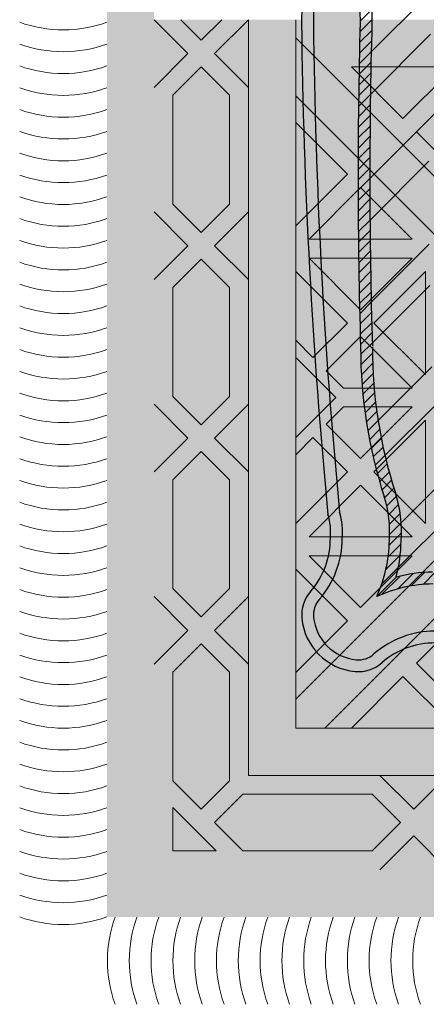
# Model space of a CAD drawing. Units: inches. Extents: x 844 to 2234, y 346 to 1084.
# Tile 52 of 93: x 1861.15 to 1866.64, y 688.07 to 701.36. Entities that reach past the tile are written whole.
import ezdxf

# ---------------------------------------------------------------- set-up
doc = ezdxf.new("R2010")
doc.units = ezdxf.units.IN
doc.header["$MEASUREMENT"] = 0
doc.layers.add('furniture', color=8, linetype='Continuous', lineweight=18)
doc.layers.add('RA-AP-01$0$INT', color=35, linetype='Continuous', lineweight=5)
doc.layers.add('RA-AP-01$0$FURN', color=3, linetype='Continuous')
doc.layers.add('RA-AP-01$0$WOOD', color=64, linetype='Continuous')

# ---------------------------------------------------------------- blocks, each defined once
blk = doc.blocks.new('A$C18D01794')
at = {"layer": 'RA-AP-01$0$INT'}
h = blk.add_hatch(color=256, dxfattribs=at)
h.paths.add_polyline_path([(4.3552, -6.1567), (4.3552, -8.0567), (5.4552, -8.0567), (5.4552, -6.1567)])
h.paths.add_polyline_path([(4.4052, -8.0067), (4.4052, -6.2067), (5.4052, -6.2067), (5.4052, -8.0067)], flags=16)
h = blk.add_hatch(color=256, dxfattribs=at)
h.paths.add_polyline_path([(4.4693, -7.0709), (4.5052, -7.035), (4.5052, -7.1067)])
h.paths.add_polyline_path([(4.4552, -7.085), (4.4769, -7.1067), (4.4335, -7.1067)])
h.paths.add_polyline_path([(4.4052, -7.035), (4.4411, -7.0709), (4.4052, -7.1067)])
h.paths.add_polyline_path([(4.4252, -6.9115), (4.4552, -6.8815), (4.4852, -6.9115), (4.4852, -7.0267), (4.4552, -7.0567), (4.4252, -7.0267)])
h.paths.add_polyline_path([(4.5052, -6.8315), (4.5052, -6.9032), (4.4693, -6.8673)])
h.paths.add_polyline_path([(4.4252, -6.7079), (4.4552, -6.6779), (4.4852, -6.7079), (4.4852, -6.8232), (4.4552, -6.8532), (4.4252, -6.8232)])
h.paths.add_polyline_path([(4.4252, -6.5044), (4.4552, -6.4744), (4.4852, -6.5044), (4.4852, -6.6196), (4.4552, -6.6496), (4.4252, -6.6196)])
h.paths.add_polyline_path([(4.4693, -6.6638), (4.5052, -6.6279), (4.5052, -6.6996)])
h.paths.add_polyline_path([(4.4052, -6.6279), (4.4411, -6.6638), (4.4052, -6.6996)])
h.paths.add_polyline_path([(4.4052, -6.4244), (4.4411, -6.4602), (4.4052, -6.4961)])
h.paths.add_polyline_path([(4.4693, -6.4602), (4.5052, -6.4244), (4.5052, -6.4961)])
h.paths.add_polyline_path([(4.4252, -6.3009), (4.4552, -6.2709), (4.4852, -6.3009), (4.4852, -6.4161), (4.4552, -6.4461), (4.4252, -6.4161)])
h.paths.add_polyline_path([(4.4252, -6.2267), (4.4711, -6.2267), (4.4252, -6.2726)])
h.paths.add_polyline_path([(4.4993, -6.2267), (4.6361, -6.2267), (4.6661, -6.2567), (4.6361, -6.2867), (4.4993, -6.2867), (4.4693, -6.2567)])
h.paths.add_polyline_path([(4.6802, -6.2709), (4.7161, -6.3067), (4.6443, -6.3067)])
h.paths.add_polyline_path([(4.6443, -6.2067), (4.7161, -6.2067), (4.6802, -6.2426)])
h.paths.add_polyline_path([(4.7243, -6.2267), (4.8611, -6.2267), (4.8911, -6.2567), (4.8611, -6.2867), (4.7243, -6.2867), (4.6943, -6.2567)])
h.paths.add_polyline_path([(4.9052, -6.2709), (4.9411, -6.3067), (4.8693, -6.3067)])
h.paths.add_polyline_path([(4.8693, -6.2067), (4.9411, -6.2067), (4.9052, -6.2426)])
h.paths.add_polyline_path([(4.9493, -6.2267), (5.0861, -6.2267), (5.1161, -6.2567), (5.0861, -6.2867), (4.9493, -6.2867), (4.9193, -6.2567)])
h.paths.add_polyline_path([(5.1302, -6.2709), (5.1661, -6.3067), (5.0943, -6.3067)])
h.paths.add_polyline_path([(5.0943, -6.2067), (5.1661, -6.2067), (5.1302, -6.2426)])
h.paths.add_polyline_path([(5.1743, -6.2267), (5.3111, -6.2267), (5.3411, -6.2567), (5.3111, -6.2867), (5.1743, -6.2867), (5.1443, -6.2567)])
h.paths.add_polyline_path([(5.3252, -6.3009), (5.3552, -6.2709), (5.3852, -6.3009), (5.3852, -6.4161), (5.3552, -6.4461), (5.3252, -6.4161)])
h.paths.add_polyline_path([(5.3393, -6.2267), (5.3852, -6.2267), (5.3852, -6.2726)])
h.paths.add_polyline_path([(5.3252, -6.5044), (5.3552, -6.4744), (5.3852, -6.5044), (5.3852, -6.6196), (5.3552, -6.6496), (5.3252, -6.6196)])
h.paths.add_polyline_path([(5.3052, -6.4244), (5.3411, -6.4602), (5.3052, -6.4961)])
h.paths.add_polyline_path([(5.3693, -6.4602), (5.4052, -6.4244), (5.4052, -6.4961)])
h.paths.add_polyline_path([(5.4052, -6.6279), (5.4052, -6.6996), (5.3693, -6.6638)])
h.paths.add_polyline_path([(5.3052, -6.6279), (5.3411, -6.6638), (5.3052, -6.6996)])
h.paths.add_polyline_path([(5.3252, -6.7079), (5.3552, -6.6779), (5.3852, -6.7079), (5.3852, -6.8232), (5.3552, -6.8532), (5.3252, -6.8232)])
h.paths.add_polyline_path([(5.3052, -6.8315), (5.3411, -6.8673), (5.3052, -6.9032)])
h.paths.add_polyline_path([(5.3252, -6.9115), (5.3552, -6.8815), (5.3852, -6.9115), (5.3852, -7.0267), (5.3552, -7.0567), (5.3252, -7.0267)])
h.paths.add_polyline_path([(5.4046, -6.8321, 0.001218), (5.4052, -6.8323), (5.4052, -6.9032), (5.3693, -6.8673)])
h.paths.add_polyline_path([(5.3693, -7.0709), (5.4052, -7.035), (5.4052, -7.1067)])
h.paths.add_polyline_path([(5.3552, -7.085), (5.3769, -7.1067), (5.3335, -7.1067)])
h.paths.add_polyline_path([(5.3052, -7.035), (5.3411, -7.0709), (5.3052, -7.1067)])
h = blk.add_hatch(color=256, dxfattribs=at)
h.paths.add_polyline_path([(4.5052, -6.6279), (4.4693, -6.6638), (4.5052, -6.6996), (4.5052, -6.8315), (4.4693, -6.8673), (4.5052, -6.9032), (4.5052, -7.035), (4.4693, -7.0709), (4.5052, -7.1067), (4.4769, -7.1067), (4.4552, -7.085), (4.4335, -7.1067), (4.4052, -7.1067), (4.4411, -7.0709), (4.4052, -7.035), (4.4052, -6.9032), (4.4411, -6.8673), (4.4052, -6.8315), (4.4052, -6.6996), (4.4411, -6.6638), (4.4052, -6.6279), (4.4052, -6.4961), (4.4411, -6.4602), (4.4052, -6.4244), (4.4052, -6.2067), (4.6443, -6.2067), (4.6802, -6.2426), (4.7161, -6.2067), (4.8693, -6.2067), (4.9052, -6.2426), (4.9411, -6.2067), (5.0943, -6.2067), (5.1302, -6.2426), (5.1661, -6.2067), (5.4052, -6.2067), (5.4052, -6.4244), (5.3693, -6.4602), (5.4052, -6.4961), (5.4052, -6.6279), (5.3693, -6.6638), (5.4052, -6.6996), (5.4052, -6.8315), (5.3693, -6.8673), (5.4052, -6.9032), (5.4052, -7.035), (5.3693, -7.0709), (5.4052, -7.1067), (5.3769, -7.1067), (5.3552, -7.085), (5.3335, -7.1067), (5.3052, -7.1067), (5.3411, -7.0709), (5.3052, -7.035), (5.3052, -6.9032), (5.3411, -6.8673), (5.3052, -6.8315), (5.3052, -6.6996), (5.3411, -6.6638), (5.3052, -6.6279), (5.3052, -6.4961), (5.3411, -6.4602), (5.3052, -6.4244), (5.3052, -6.3067), (5.1661, -6.3067), (5.1302, -6.2709), (5.0943, -6.3067), (4.9411, -6.3067), (4.9052, -6.2709), (4.8693, -6.3067), (4.7161, -6.3067), (4.6802, -6.2709), (4.6443, -6.3067), (4.5052, -6.3067), (4.5052, -6.4244), (4.4693, -6.4602), (4.5052, -6.4961)])
h.paths.add_polyline_path([(4.4852, -6.5044), (4.4552, -6.4744), (4.4252, -6.5044), (4.4252, -6.6196), (4.4552, -6.6496), (4.4852, -6.6196)], flags=16)
h.paths.add_polyline_path([(4.4552, -6.4461), (4.4852, -6.4161), (4.4852, -6.3009), (4.4552, -6.2709), (4.4252, -6.3009), (4.4252, -6.4161)], flags=16)
h.paths.add_polyline_path([(4.4552, -6.6779), (4.4252, -6.7079), (4.4252, -6.8232), (4.4552, -6.8532), (4.4852, -6.8232), (4.4852, -6.7079)], flags=16)
h.paths.add_polyline_path([(4.4993, -6.2867), (4.6361, -6.2867), (4.6661, -6.2567), (4.6361, -6.2267), (4.4993, -6.2267), (4.4693, -6.2567)], flags=16)
h.paths.add_polyline_path([(4.4252, -6.2726), (4.4711, -6.2267), (4.4252, -6.2267)], flags=16)
h.paths.add_polyline_path([(4.4552, -6.8815), (4.4252, -6.9115), (4.4252, -7.0267), (4.4552, -7.0567), (4.4852, -7.0267), (4.4852, -6.9115)], flags=16)
h.paths.add_polyline_path([(4.7243, -6.2867), (4.8611, -6.2867), (4.8911, -6.2567), (4.8611, -6.2267), (4.7243, -6.2267), (4.6943, -6.2567)], flags=16)
h.paths.add_polyline_path([(4.9193, -6.2567), (4.9493, -6.2867), (5.0861, -6.2867), (5.1161, -6.2567), (5.0861, -6.2267), (4.9493, -6.2267)], flags=16)
h.paths.add_polyline_path([(5.1443, -6.2567), (5.1743, -6.2867), (5.3111, -6.2867), (5.3411, -6.2567), (5.3111, -6.2267), (5.1743, -6.2267)], flags=16)
h.paths.add_polyline_path([(5.3252, -6.6196), (5.3552, -6.6496), (5.3852, -6.6196), (5.3852, -6.5044), (5.3552, -6.4744), (5.3252, -6.5044)], flags=16)
h.paths.add_polyline_path([(5.3252, -6.4161), (5.3552, -6.4461), (5.3852, -6.4161), (5.3852, -6.3009), (5.3552, -6.2709), (5.3252, -6.3009)], flags=16)
h.paths.add_polyline_path([(5.3252, -6.7079), (5.3252, -6.8232), (5.3552, -6.8532), (5.3852, -6.8232), (5.3852, -6.7079), (5.3552, -6.6779)], flags=16)
h.paths.add_polyline_path([(5.3252, -6.9115), (5.3252, -7.0267), (5.3552, -7.0567), (5.3852, -7.0267), (5.3852, -6.9115), (5.3552, -6.8815)], flags=16)
h.paths.add_polyline_path([(5.3393, -6.2267), (5.3852, -6.2726), (5.3852, -6.2267)], flags=16)
for points in [[(4.5052, -6.3067), (5.3052, -6.3067), (5.3052, -7.1067), (5.2552, -7.1067), (5.2552, -6.3567), (4.5552, -6.3567), (4.5552, -7.1067), (4.5052, -7.1067)], [(4.4052, -6.9032), (4.4411, -6.8673), (4.4052, -6.8315)]]:
    blk.add_hatch(color=256, dxfattribs=at).paths.add_polyline_path(points)
h = blk.add_hatch(color=256, dxfattribs=at)
h.paths.add_polyline_path([(4.5859, -6.3567), (4.5552, -6.3567), (4.5552, -6.3874), (4.8745, -6.7067), (4.9052, -6.676)])
h.paths.add_polyline_path([(5.2552, -6.3874), (5.2552, -6.3567), (5.2245, -6.3567), (4.9052, -6.676), (4.9359, -6.7067)])
h.paths.add_polyline_path([(4.9359, -6.7067), (4.9052, -6.7374), (5.2552, -7.0874), (5.2552, -7.026)])
h.paths.add_polyline_path([(4.5552, -7.026), (4.5552, -7.0874), (4.9052, -6.7374), (4.8745, -6.7067)])
h = blk.add_hatch(color=256, dxfattribs=at)
h.paths.add_polyline_path([(4.5859, -6.3567), (4.6142, -6.3567), (4.6688, -6.4114), (4.7235, -6.3567), (4.7718, -6.3567), (4.8264, -6.4114), (4.8628, -6.375), (4.8445, -6.3567), (4.8628, -6.3567), (4.9052, -6.3991), (4.9476, -6.3567), (4.9659, -6.3567), (4.9476, -6.375), (4.984, -6.4114), (5.0386, -6.3567), (5.0869, -6.3567), (5.1416, -6.4114), (5.1962, -6.3567), (5.2245, -6.3567), (4.9052, -6.676)])
h.paths.add_polyline_path([(4.8952, -6.6377), (4.8952, -6.5284), (4.8406, -6.5831)], flags=16)
h.paths.add_polyline_path([(4.9152, -6.6377), (4.9699, -6.5831), (4.9152, -6.5284)], flags=16)
h.paths.add_polyline_path([(4.8264, -6.5689), (4.8811, -6.5143), (4.7718, -6.5143)], flags=16)
h.paths.add_polyline_path([(4.984, -6.5689), (5.0386, -6.5143), (4.9293, -6.5143)], flags=16)
h.paths.add_polyline_path([(4.8811, -6.4943), (4.8264, -6.4396), (4.7718, -6.4943)], flags=16)
h.paths.add_polyline_path([(4.9293, -6.4943), (5.0386, -6.4943), (4.984, -6.4396)], flags=16)
h.paths.add_polyline_path([(4.8952, -6.4801), (4.8952, -6.4074), (4.8769, -6.3891), (4.8406, -6.4255)], flags=16)
h.paths.add_polyline_path([(4.9152, -6.4801), (4.9699, -6.4255), (4.9335, -6.3891), (4.9152, -6.4074)], flags=16)
h.paths.add_polyline_path([(4.7576, -6.4801), (4.8123, -6.4255), (4.7576, -6.3709)], flags=16)
h.paths.add_polyline_path([(4.7376, -6.4801), (4.7376, -6.3709), (4.683, -6.4255)], flags=16)
h.paths.add_polyline_path([(5.0528, -6.4801), (5.0528, -6.3709), (4.9981, -6.4255)], flags=16)
h.paths.add_polyline_path([(5.0728, -6.4801), (5.1274, -6.4255), (5.0728, -6.3709)], flags=16)
h.paths.add_polyline_path([(4.9359, -6.7067), (5.2552, -6.3874), (5.2552, -6.4157), (5.2006, -6.4704), (5.2552, -6.525), (5.2552, -6.5733), (5.2006, -6.6279), (5.2369, -6.6643), (5.2552, -6.646), (5.2552, -6.6643), (5.2128, -6.7067), (5.2552, -6.7491), (5.2552, -6.7674), (5.2369, -6.7491), (5.2006, -6.7855), (5.2552, -6.8401), (5.2552, -6.8884), (5.2006, -6.9431), (5.2552, -6.9977), (5.2552, -7.026)])
h.paths.add_polyline_path([(5.043, -6.7855), (5.0976, -6.8401), (5.0976, -6.7309)], flags=16)
h.paths.add_polyline_path([(5.0288, -6.7714), (5.0835, -6.7167), (4.9742, -6.7167)], flags=16)
h.paths.add_polyline_path([(5.1176, -6.8401), (5.1723, -6.7855), (5.1176, -6.7309)], flags=16)
h.paths.add_polyline_path([(5.0835, -6.6967), (5.0288, -6.6421), (4.9742, -6.6967)], flags=16)
h.paths.add_polyline_path([(5.1318, -6.8543), (5.1864, -6.7996), (5.2411, -6.8543)], flags=17)
h.paths.add_polyline_path([(5.1318, -6.7167), (5.1864, -6.7714), (5.2228, -6.735), (5.2045, -6.7167)], flags=16)
h.paths.add_polyline_path([(5.0976, -6.6826), (5.0976, -6.5733), (5.043, -6.6279)], flags=16)
h.paths.add_polyline_path([(5.1318, -6.8743), (5.2411, -6.8743), (5.1864, -6.9289)], flags=17)
h.paths.add_polyline_path([(5.1318, -6.6967), (5.2045, -6.6967), (5.2228, -6.6784), (5.1864, -6.6421)], flags=16)
h.paths.add_polyline_path([(5.1176, -6.6826), (5.1723, -6.6279), (5.1176, -6.5733)], flags=16)
h.paths.add_polyline_path([(5.1864, -6.6138), (5.2411, -6.5591), (5.1318, -6.5591)], flags=16)
h.paths.add_polyline_path([(5.1318, -6.5391), (5.2411, -6.5391), (5.1864, -6.4845)], flags=16)
h.paths.add_polyline_path([(5.2552, -7.0874), (5.2552, -7.1067), (4.5552, -7.1067), (4.5552, -7.0874), (4.9052, -6.7374)])
h.paths.add_polyline_path([(4.984, -6.8445), (4.9293, -6.8991), (5.0386, -6.8991)], flags=16)
h.paths.add_polyline_path([(4.9699, -6.8304), (4.9152, -6.7757), (4.9152, -6.885)], flags=16)
h.paths.add_polyline_path([(4.9293, -6.9191), (4.984, -6.9738), (5.0386, -6.9191)], flags=16)
h.paths.add_polyline_path([(5.0528, -6.9333), (4.9981, -6.9879), (5.0528, -7.0426)], flags=16)
h.paths.add_polyline_path([(5.0728, -6.9333), (5.0728, -7.0426), (5.1274, -6.9879)], flags=16)
h.paths.add_polyline_path([(4.8952, -6.7757), (4.8406, -6.8304), (4.8952, -6.885)], flags=16)
h.paths.add_polyline_path([(4.9152, -6.9333), (4.9152, -7.006), (4.9335, -7.0243), (4.9699, -6.9879)], flags=16)
h.paths.add_polyline_path([(4.8811, -6.8991), (4.8264, -6.8445), (4.7718, -6.8991)], flags=16)
h.paths.add_polyline_path([(4.8952, -6.9333), (4.8406, -6.9879), (4.8769, -7.0243), (4.8952, -7.006)], flags=16)
h.paths.add_polyline_path([(4.984, -7.0021), (4.9476, -7.0384), (4.9659, -7.0567), (5.0386, -7.0567)], flags=16)
h.paths.add_polyline_path([(4.8811, -6.9191), (4.7718, -6.9191), (4.8264, -6.9738)], flags=16)
h.paths.add_polyline_path([(4.9052, -7.0143), (4.8628, -7.0567), (4.9476, -7.0567)], flags=16)
h.paths.add_polyline_path([(5.1416, -7.0021), (5.0869, -7.0567), (5.1962, -7.0567)], flags=16)
h.paths.add_polyline_path([(4.8264, -7.0021), (4.7718, -7.0567), (4.8445, -7.0567), (4.8628, -7.0384)], flags=16)
h.paths.add_polyline_path([(4.8123, -6.9879), (4.7576, -6.9333), (4.7576, -7.0426)], flags=16)
h.paths.add_polyline_path([(4.7376, -6.9333), (4.683, -6.9879), (4.7376, -7.0426)], flags=16)
h.paths.add_polyline_path([(4.7235, -7.0567), (4.6688, -7.0021), (4.6142, -7.0567)], flags=16)
h.paths.add_polyline_path([(4.5976, -6.7067), (4.5552, -6.6643), (4.5552, -6.646), (4.5735, -6.6643), (4.6099, -6.6279), (4.5552, -6.5733), (4.5552, -6.525), (4.6099, -6.4704), (4.5552, -6.4157), (4.5552, -6.3874), (4.8745, -6.7067), (4.5552, -7.026), (4.5552, -6.9977), (4.6099, -6.9431), (4.5552, -6.8884), (4.5552, -6.8401), (4.6099, -6.7855), (4.5735, -6.7491), (4.5552, -6.7674), (4.5552, -6.7491)])
h.paths.add_polyline_path([(4.7128, -6.7309), (4.7128, -6.8401), (4.7674, -6.7855)], flags=16)
h.paths.add_polyline_path([(4.7269, -6.7167), (4.7816, -6.7714), (4.8362, -6.7167)], flags=16)
h.paths.add_polyline_path([(4.6928, -6.7309), (4.6381, -6.7855), (4.6928, -6.8401)], flags=16)
h.paths.add_polyline_path([(4.7269, -6.6967), (4.8362, -6.6967), (4.7816, -6.6421)], flags=16)
h.paths.add_polyline_path([(4.6786, -6.7167), (4.6059, -6.7167), (4.5876, -6.735), (4.624, -6.7714)], flags=16)
h.paths.add_polyline_path([(4.7128, -6.6826), (4.7674, -6.6279), (4.7128, -6.5733)], flags=16)
h.paths.add_polyline_path([(4.6786, -6.6967), (4.624, -6.6421), (4.5876, -6.6784), (4.6059, -6.6967)], flags=16)
h.paths.add_polyline_path([(4.6928, -6.6826), (4.6928, -6.5733), (4.6381, -6.6279)], flags=16)
h.paths.add_polyline_path([(4.624, -6.7996), (4.6786, -6.8543), (4.5693, -6.8543)], flags=17)
h.paths.add_polyline_path([(4.624, -6.6138), (4.6786, -6.5591), (4.5693, -6.5591)], flags=16)
h.paths.add_polyline_path([(4.6786, -6.8743), (4.624, -6.9289), (4.5693, -6.8743)], flags=17)
h.paths.add_polyline_path([(4.6786, -6.5391), (4.624, -6.4845), (4.5693, -6.5391)], flags=16)
h = blk.add_hatch(color=256, dxfattribs=at)
h.paths.add_polyline_path([(4.9699, -6.5831), (4.9152, -6.6377), (4.9152, -6.5284)])
h.paths.add_polyline_path([(4.8952, -6.6377), (4.8406, -6.5831), (4.8952, -6.5284)])
h.paths.add_polyline_path([(4.8264, -6.5689), (4.7718, -6.5143), (4.8811, -6.5143)])
h.paths.add_polyline_path([(4.8811, -6.4943), (4.7718, -6.4943), (4.8264, -6.4396)])
h.paths.add_polyline_path([(4.8952, -6.4801), (4.8406, -6.4255), (4.8769, -6.3891), (4.8952, -6.4074)])
h.paths.add_polyline_path([(4.8628, -6.375), (4.8264, -6.4114), (4.7718, -6.3567), (4.8445, -6.3567)])
h.paths.add_polyline_path([(4.8123, -6.4255), (4.7576, -6.4801), (4.7576, -6.3709)])
h.paths.add_polyline_path([(4.7376, -6.4801), (4.683, -6.4255), (4.7376, -6.3709)])
h.paths.add_polyline_path([(4.6688, -6.4114), (4.6142, -6.3567), (4.7235, -6.3567)])
h.paths.add_polyline_path([(4.9052, -6.3991), (4.8628, -6.3567), (4.9476, -6.3567)])
h.paths.add_polyline_path([(4.9152, -6.4801), (4.9152, -6.4074), (4.9335, -6.3891), (4.9699, -6.4255)])
h.paths.add_polyline_path([(5.0386, -6.4943), (4.9293, -6.4943), (4.984, -6.4396)])
h.paths.add_polyline_path([(4.984, -6.5689), (4.9293, -6.5143), (5.0386, -6.5143)])
h.paths.add_polyline_path([(5.0528, -6.4801), (4.9981, -6.4255), (5.0528, -6.3709)])
h.paths.add_polyline_path([(4.984, -6.4114), (4.9476, -6.375), (4.9659, -6.3567), (5.0386, -6.3567)])
h.paths.add_polyline_path([(5.1274, -6.4255), (5.0728, -6.4801), (5.0728, -6.3709)])
h.paths.add_polyline_path([(5.1416, -6.4114), (5.0869, -6.3567), (5.1962, -6.3567)])
h = blk.add_hatch(color=256, dxfattribs=at)
h.paths.add_polyline_path([(4.7816, -6.7714), (4.8362, -6.7167), (4.7269, -6.7167)])
h.paths.add_polyline_path([(4.8362, -6.6967), (4.7816, -6.6421), (4.7269, -6.6967)])
h.paths.add_polyline_path([(4.7674, -6.6279), (4.7128, -6.5733), (4.7128, -6.6826)])
h.paths.add_polyline_path([(4.6928, -6.6826), (4.6928, -6.5733), (4.6381, -6.6279)])
h.paths.add_polyline_path([(4.6786, -6.6967), (4.624, -6.6421), (4.5876, -6.6784), (4.6059, -6.6967)])
h.paths.add_polyline_path([(4.5735, -6.6643), (4.6099, -6.6279), (4.5552, -6.5733), (4.5552, -6.646)])
h.paths.add_polyline_path([(4.624, -6.6138), (4.6786, -6.5591), (4.5693, -6.5591)])
h.paths.add_polyline_path([(4.6786, -6.5391), (4.624, -6.4845), (4.5693, -6.5391)])
h.paths.add_polyline_path([(4.6099, -6.4704), (4.5552, -6.4157), (4.5552, -6.525)])
h.paths.add_polyline_path([(4.5976, -6.7067), (4.5552, -6.6643), (4.5552, -6.7491)])
h.paths.add_polyline_path([(4.6786, -6.7167), (4.6059, -6.7167), (4.5876, -6.735), (4.624, -6.7714)])
h.paths.add_polyline_path([(4.6928, -6.8401), (4.6928, -6.7309), (4.6381, -6.7855)])
h.paths.add_polyline_path([(4.7674, -6.7855), (4.7128, -6.7309), (4.7128, -6.8401)])
h.paths.add_polyline_path([(4.6786, -6.8543), (4.624, -6.7996), (4.5693, -6.8543)])
h.paths.add_polyline_path([(4.6099, -6.7855), (4.5735, -6.7491), (4.5552, -6.7674), (4.5552, -6.8401)])
h.paths.add_polyline_path([(4.624, -6.9289), (4.6786, -6.8743), (4.5693, -6.8743)])
h.paths.add_polyline_path([(4.6099, -6.9431), (4.5552, -6.8884), (4.5552, -6.9977)])
h = blk.add_hatch(color=256, dxfattribs=at)
h.paths.add_polyline_path([(4.8952, -6.7757), (4.8406, -6.8304), (4.8952, -6.885)])
h.paths.add_polyline_path([(4.9152, -6.885), (4.9699, -6.8304), (4.9152, -6.7757)])
h.paths.add_polyline_path([(5.0386, -6.8991), (4.984, -6.8445), (4.9293, -6.8991)])
h.paths.add_polyline_path([(4.9293, -6.9191), (4.984, -6.9738), (5.0386, -6.9191)])
h.paths.add_polyline_path([(4.9152, -6.9333), (4.9152, -7.006), (4.9335, -7.0243), (4.9699, -6.9879)])
h.paths.add_polyline_path([(5.0386, -7.0567), (4.984, -7.0021), (4.9476, -7.0384), (4.9659, -7.0567)])
h.paths.add_polyline_path([(5.0528, -7.0426), (5.0528, -6.9333), (4.9981, -6.9879)])
h.paths.add_polyline_path([(5.0728, -7.0426), (5.1274, -6.9879), (5.0728, -6.9333)])
h.paths.add_polyline_path([(5.1416, -7.0021), (5.0869, -7.0567), (5.1962, -7.0567)])
h.paths.add_polyline_path([(4.9476, -7.0567), (4.9052, -7.0143), (4.8628, -7.0567)])
h.paths.add_polyline_path([(4.8406, -6.9879), (4.8769, -7.0243), (4.8952, -7.006), (4.8952, -6.9333)])
h.paths.add_polyline_path([(4.8811, -6.9191), (4.7718, -6.9191), (4.8264, -6.9738)])
h.paths.add_polyline_path([(4.8811, -6.8991), (4.8264, -6.8445), (4.7718, -6.8991)])
h.paths.add_polyline_path([(4.7576, -7.0426), (4.8123, -6.9879), (4.7576, -6.9333)])
h.paths.add_polyline_path([(4.8264, -7.0021), (4.7718, -7.0567), (4.8445, -7.0567), (4.8628, -7.0384)])
h.paths.add_polyline_path([(4.7376, -7.0426), (4.7376, -6.9333), (4.683, -6.9879)])
h.paths.add_polyline_path([(4.6688, -7.0021), (4.6142, -7.0567), (4.7235, -7.0567)])
for p, q in [((4.6443, -6.2067), (4.6802, -6.2426)), ((4.7161, -6.2067), (4.6802, -6.2426)), ((4.4711, -6.2267), (4.4252, -6.2726)), ((4.4252, -6.2726), (4.4252, -6.2267)), ((4.4711, -6.2267), (4.4252, -6.2267)), ((4.4993, -6.2267), (4.4693, -6.2567)), ((4.6361, -6.2267), (4.4993, -6.2267)), ((4.6361, -6.2267), (4.6661, -6.2567)), ((4.4993, -6.2867), (4.4693, -6.2567)), ((4.6361, -6.2867), (4.6661, -6.2567)), ((4.4252, -6.3009), (4.4552, -6.2709)), ((4.4852, -6.3009), (4.4552, -6.2709)), ((4.6443, -6.3067), (4.6802, -6.2709)), ((4.7161, -6.3067), (4.6802, -6.2709)), ((4.6361, -6.2867), (4.4993, -6.2867)), ((4.4252, -6.4161), (4.4252, -6.3009)), ((4.4852, -6.3009), (4.4852, -6.4161)), ((5.2672, -6.3067), (4.5432, -6.3067)), ((5.2672, -6.3067), (4.5432, -6.3067)), ((4.5552, -6.3567), (5.2552, -6.3567)), ((4.5552, -7.1067), (4.5552, -6.3567)), ((4.9052, -6.676), (4.5859, -6.3567)), ((4.6142, -6.3567), (4.6688, -6.4114)), ((4.7235, -6.3567), (4.6688, -6.4114)), ((4.7376, -6.3709), (4.683, -6.4255)), ((4.8745, -6.7067), (4.5552, -6.3874)), ((4.4552, -6.4461), (4.4252, -6.4161)), ((4.4552, -6.4461), (4.4852, -6.4161)), ((4.5552, -6.4157), (4.6099, -6.4704)), ((4.4411, -6.4602), (4.4052, -6.4244)), ((4.4693, -6.4602), (4.5052, -6.4244)), ((4.683, -6.4255), (4.7376, -6.4801)), ((4.4052, -6.4961), (4.4411, -6.4602)), ((4.5052, -6.4961), (4.4693, -6.4602)), ((4.5552, -6.525), (4.6099, -6.4704)), ((4.4252, -6.5044), (4.4552, -6.4744)), ((4.4852, -6.5044), (4.4552, -6.4744)), ((4.5693, -6.5391), (4.624, -6.4845)), ((4.624, -6.4845), (4.6786, -6.5391)), ((4.4252, -6.6196), (4.4252, -6.5044)), ((4.4852, -6.6196), (4.4852, -6.5044)), ((4.6786, -6.5391), (4.5693, -6.5391)), ((4.5693, -6.5591), (4.624, -6.6138)), ((4.6786, -6.5591), (4.5693, -6.5591)), ((4.6786, -6.5591), (4.624, -6.6138)), ((4.5552, -6.646), (4.5552, -6.5733)), ((4.5552, -6.5733), (4.6099, -6.6279)), ((4.6928, -6.5733), (4.6381, -6.6279)), ((4.6928, -6.5733), (4.6928, -6.6826)), ((4.4052, -6.6279), (4.4411, -6.6638)), ((4.4252, -6.6196), (4.4552, -6.6496)), ((4.4852, -6.6196), (4.4552, -6.6496)), ((4.5052, -6.6279), (4.4693, -6.6638)), ((4.6099, -6.6279), (4.5735, -6.6643)), ((4.6928, -6.6826), (4.6381, -6.6279)), ((4.5552, -6.646), (4.5735, -6.6643)), ((4.624, -6.6421), (4.5876, -6.6784)), ((4.6786, -6.6967), (4.624, -6.6421)), ((4.4052, -6.6996), (4.4411, -6.6638)), ((4.5052, -6.6996), (4.4693, -6.6638)), ((4.5552, -6.7491), (4.5552, -6.6643)), ((4.5976, -6.7067), (4.5552, -6.6643)), ((4.4252, -6.7079), (4.4552, -6.6779)), ((4.4852, -6.7079), (4.4552, -6.6779)), ((4.6059, -6.6967), (4.5876, -6.6784)), ((4.6059, -6.6967), (4.6786, -6.6967)), ((4.4252, -6.8232), (4.4252, -6.7079)), ((4.4852, -6.8232), (4.4852, -6.7079)), ((4.8745, -6.7067), (4.5552, -7.026)), ((4.5976, -6.7067), (4.5552, -6.7491)), ((4.6059, -6.7167), (4.5876, -6.735)), ((4.6059, -6.7167), (4.6786, -6.7167)), ((4.6786, -6.7167), (4.624, -6.7714)), ((4.6928, -6.7309), (4.6381, -6.7855)), ((4.6928, -6.8401), (4.6928, -6.7309)), ((4.9052, -6.7374), (4.5552, -7.0874)), ((4.624, -6.7714), (4.5876, -6.735)), ((4.5735, -6.7491), (4.5552, -6.7674)), ((4.5552, -6.7674), (4.5735, -6.7491)), ((4.6099, -6.7855), (4.5735, -6.7491)), ((4.5552, -6.7674), (4.5552, -6.8401)), ((4.5552, -6.8401), (4.6099, -6.7855)), ((4.6928, -6.8401), (4.6381, -6.7855)), ((4.5693, -6.8543), (4.624, -6.7996)), ((4.6786, -6.8543), (4.624, -6.7996)), ((4.4252, -6.8232), (4.4552, -6.8532)), ((4.4852, -6.8232), (4.4552, -6.8532)), ((4.4052, -6.8315), (4.4411, -6.8673)), ((4.5052, -6.8315), (4.4693, -6.8673)), ((4.6786, -6.8543), (4.5693, -6.8543)), ((4.4052, -6.9032), (4.4411, -6.8673)), ((4.5052, -6.9032), (4.4693, -6.8673)), ((4.5693, -6.8743), (4.624, -6.9289)), ((4.6786, -6.8743), (4.5693, -6.8743)), ((4.624, -6.9289), (4.6786, -6.8743)), ((4.4252, -6.9115), (4.4552, -6.8815)), ((4.4852, -6.9115), (4.4552, -6.8815)), ((4.5552, -6.8884), (4.6099, -6.9431)), ((4.5552, -6.8884), (4.5552, -6.9977)), ((4.4252, -6.9115), (4.4252, -7.0267)), ((4.4852, -6.9115), (4.4852, -7.0267)), ((4.683, -6.9879), (4.7376, -6.9333)), ((4.5552, -6.9977), (4.6099, -6.9431)), ((4.7376, -7.0426), (4.683, -6.9879)), ((4.6142, -7.0567), (4.6688, -7.0021)), ((4.7235, -7.0567), (4.6688, -7.0021)), ((4.4052, -7.035), (4.4411, -7.0709)), ((4.4252, -7.0267), (4.4552, -7.0567)), ((4.4852, -7.0267), (4.4552, -7.0567)), ((4.5052, -7.035), (4.4693, -7.0709)), ((4.7235, -7.0567), (4.6142, -7.0567)), ((4.4411, -7.0709), (4.4052, -7.1067)), ((4.4693, -7.0709), (4.5052, -7.1067)), ((4.4552, -7.085), (4.4335, -7.1067)), ((4.4552, -7.085), (4.4769, -7.1067))]:
    blk.add_line(p, q, dxfattribs=at)
blk.add_lwpolyline([(5.3052, -7.1067), (5.3052, -6.3067), (4.5052, -6.3067), (4.5052, -7.1067)], dxfattribs=at)
for centre, start, end in [((4.4922, -6.1105), 160.2038, 199.7962), ((4.5153, -6.1105), 160.2038, 199.7962), ((4.5384, -6.1105), 160.2038, 199.7962), ((4.5615, -6.1105), 160.2038, 199.7962), ((4.5846, -6.1105), 160.2038, 199.7962), ((4.6077, -6.1105), 160.2038, 199.7962), ((4.6308, -6.1105), 160.2038, 199.7962), ((4.6539, -6.1105), 160.2038, 199.7962), ((4.677, -6.1105), 160.2038, 199.7962), ((4.7001, -6.1105), 160.2038, 199.7962), ((4.7232, -6.1105), 160.2038, 199.7962), ((4.7463, -6.1105), 160.2038, 199.7962), ((4.7694, -6.1105), 160.2038, 199.7962), ((4.7925, -6.1105), 160.2038, 199.7962), ((4.8156, -6.1105), 160.2038, 199.7962), ((4.309, -6.2852), 70.2038, 109.7962), ((4.309, -6.3083), 70.2038, 109.7962), ((4.309, -6.3314), 70.2038, 109.7962), ((4.309, -6.3545), 70.2038, 109.7962), ((4.309, -6.3776), 70.2038, 109.7962), ((4.309, -6.4007), 70.2038, 109.7962), ((4.309, -6.4238), 70.2038, 109.7962), ((4.309, -6.4469), 70.2038, 109.7962), ((4.309, -6.47), 70.2038, 109.7962), ((4.309, -6.4931), 70.2038, 109.7962), ((4.309, -6.5162), 70.2038, 109.7962), ((4.309, -6.5393), 70.2038, 109.7962), ((4.309, -6.5624), 70.2038, 109.7962), ((4.309, -6.5855), 70.2038, 109.7962), ((4.309, -6.6086), 70.2038, 109.7962), ((4.309, -6.6317), 70.2038, 109.7962), ((4.309, -6.6548), 70.2038, 109.7962), ((4.309, -6.6779), 70.2038, 109.7962), ((4.309, -6.701), 70.2038, 109.7962), ((4.309, -6.7241), 70.2038, 109.7962), ((4.309, -6.7472), 70.2038, 109.7962), ((4.309, -6.7703), 70.2038, 109.7962), ((4.309, -6.7934), 70.2038, 109.7962), ((4.309, -6.7934), 70.2038, 109.7962), ((4.309, -6.8165), 70.2038, 109.7962), ((4.309, -6.8396), 70.2038, 109.7962), ((4.309, -6.8627), 70.2038, 109.7962), ((4.309, -6.8858), 70.2038, 109.7962), ((4.309, -6.9089), 70.2038, 109.7962), ((4.309, -6.932), 70.2038, 109.7962), ((4.309, -6.9551), 70.2038, 109.7962), ((4.309, -6.9782), 70.2038, 109.7962), ((4.309, -7.0013), 70.2038, 109.7962), ((4.309, -7.0244), 70.2038, 109.7962), ((4.309, -7.0475), 70.2038, 109.7962), ((4.309, -7.0706), 70.2038, 109.7962), ((4.309, -7.0937), 70.2038, 109.7962), ((4.309, -7.1168), 70.2038, 109.7962), ((4.309, -7.1399), 70.2038, 109.7962), ((4.309, -7.163), 70.2038, 109.7962), ((4.309, -7.1861), 70.2038, 109.7962), ((4.309, -7.2092), 70.2038, 109.7962), ((4.309, -7.2323), 70.2038, 109.7962)]:
    blk.add_arc(centre, 0.1364, start, end, dxfattribs=at)
blk = doc.blocks.new('A$C32926AE1')
at = {"layer": 'RA-AP-01$0$WOOD'}
h = blk.add_hatch(color=256, dxfattribs=at)
h.dxf.hatch_style = 1
h.paths.add_polyline_path([(5.15743, 4.57348, -0.100949), (5.1554, 4.59337, -0.184266), (5.17225, 4.6388, 0.205661), (5.17956, 4.66132, 0.361434), (5.13435, 4.70652, 0.205661), (5.11183, 4.69921, -0.184266), (5.0664, 4.68237, -0.105531), (5.04566, 4.68467, 0.156764), (4.76389, 4.68467, -0.105531), (4.74314, 4.68237, -0.184266), (4.69771, 4.69921, 0.205661), (4.67519, 4.70652, 0.361434), (4.62998, 4.66132, 0.205661), (4.63729, 4.6388, -0.184266), (4.65414, 4.59337, -0.100949), (4.65211, 4.57348, 0.02141), (4.62975, 4.15671, 0.02141), (4.65211, 3.73994, -0.100949), (4.65414, 3.72006, -0.184266), (4.63729, 3.67463, 0.205661), (4.62998, 3.65211, 0.361434), (4.67519, 3.6069, 0.205661), (4.69771, 3.61421, -0.184266), (4.74314, 3.63106, -0.105531), (4.76389, 3.62875, 0.156764), (5.04566, 3.62875, -0.105531), (5.0664, 3.63106, -0.184266), (5.11183, 3.61421, 0.205661), (5.13435, 3.6069, 0.361434), (5.17956, 3.65211, 0.205661), (5.17225, 3.67463, -0.184266), (5.1554, 3.72006, -0.100949), (5.15743, 3.73994, 0.02141), (5.17979, 4.15671, 0.02141)])
h.paths.add_polyline_path([(4.63975, 4.15671, 0.021354), (4.66197, 3.74189, -0.094076), (4.66414, 3.71961, -0.182482), (4.64481, 3.66804, 0.205661), (4.63994, 3.65302, 0.361434), (4.67611, 3.61686, 0.205661), (4.69112, 3.62173, -0.182482), (4.7427, 3.64106, -0.102989), (4.76699, 3.63826, 0.156709), (5.04255, 3.63826, -0.102989), (5.06685, 3.64106, -0.182482), (5.11842, 3.62173, 0.205661), (5.13344, 3.61686, 0.361434), (5.1696, 3.65302, 0.205661), (5.16473, 3.66804, -0.182482), (5.1454, 3.71961, -0.094076), (5.14757, 3.74189, 0.021354), (5.16979, 4.15671, 0.021354), (5.14757, 4.57154, -0.094076), (5.1454, 4.59381, -0.182482), (5.16473, 4.64539, 0.205661), (5.1696, 4.6604, 0.361434), (5.13344, 4.69657, 0.205661), (5.11842, 4.69169, -0.182482), (5.06685, 4.67236, -0.102989), (5.04255, 4.67517, 0.156709), (4.76699, 4.67517, -0.102989), (4.7427, 4.67236, -0.182482), (4.69112, 4.69169, 0.205661), (4.67611, 4.69657, 0.361434), (4.63994, 4.6604, 0.205661), (4.64481, 4.64539, -0.182482), (4.66414, 4.59381, -0.094076), (4.66197, 4.57154, 0.021354)], flags=16)
h.paths.add_polyline_path([(5.12979, 4.43217, -0.014166), (5.13015, 4.15693, -0.014166), (5.12979, 3.88169, -0.078525), (5.1098, 3.75514, 0.094597), (5.10541, 3.7179, 0.104317), (5.11607, 3.67039, 0.104317), (5.06856, 3.68105, 0.094597), (5.03132, 3.67666, -0.158024), (4.77823, 3.67666, 0.094597), (4.74098, 3.68105, 0.104317), (4.69347, 3.67039, 0.104317), (4.70413, 3.7179, 0.094597), (4.69975, 3.75514, -0.078525), (4.67975, 3.88169, -0.014166), (4.67939, 4.15693, -0.014166), (4.67975, 4.43217, -0.078525), (4.69975, 4.55871, 0.094597), (4.70413, 4.59596, 0.104317), (4.69347, 4.64347, 0.104317), (4.74098, 4.6328, 0.094597), (4.77823, 4.63719, -0.158024), (5.03132, 4.63719, 0.094597), (5.06856, 4.6328, 0.104317), (5.11607, 4.64347, 0.104317), (5.10541, 4.59596, 0.094597), (5.1098, 4.55871, -0.078525)], flags=0)
h.paths.add_polyline_path([(5.11979, 4.43226, -0.0142), (5.12016, 4.15693, -0.0142), (5.11979, 3.8816, -0.078489), (5.10027, 3.75819, 0.094014), (5.09541, 3.71748, 0.060627), (5.09962, 3.68684, 0.060627), (5.06898, 3.69105, 0.094014), (5.02827, 3.68619, -0.158071), (4.78127, 3.68619, 0.094014), (4.74056, 3.69105, 0.060627), (4.70993, 3.68684, 0.060627), (4.71413, 3.71748, 0.094014), (4.70927, 3.75819, -0.078489), (4.68975, 3.8816, -0.0142), (4.68939, 4.15693, -0.0142), (4.68975, 4.43226, -0.078489), (4.70927, 4.55566, 0.094014), (4.71413, 4.59638, 0.060627), (4.70993, 4.62701, 0.060627), (4.74056, 4.62281, 0.094014), (4.78127, 4.62767, -0.158071), (5.02827, 4.62767, 0.094014), (5.06898, 4.62281, 0.060627), (5.09962, 4.62701, 0.060627), (5.09541, 4.59638, 0.094014), (5.10027, 4.55566, -0.078489)], flags=0)
h.paths.add_polyline_path([(5.06979, 4.43022, -0.014242), (5.07017, 4.15693, -0.014242), (5.06979, 3.88364, -0.080061), (5.05266, 3.77346, 0.052642), (5.04591, 3.74055, 0.052642), (5.013, 3.7338, -0.158303), (4.79655, 3.7338, 0.052642), (4.76363, 3.74055, 0.052642), (4.75688, 3.77346, -0.080061), (4.73975, 3.88364, -0.014242), (4.73937, 4.15693, -0.014242), (4.73975, 4.43022, -0.080061), (4.75688, 4.54039, 0.052642), (4.76363, 4.5733, 0.052642), (4.79655, 4.58006, -0.158303), (5.013, 4.58006, 0.052642), (5.04591, 4.5733, 0.052642), (5.05266, 4.54039, -0.080061)], flags=0)
h.paths.add_polyline_path([(5.04979, 4.43038, -0.01431), (5.05018, 4.15693, -0.01431), (5.04979, 3.88347, -0.080069), (5.03362, 3.77958, 0.030626), (5.02824, 3.75822, 0.030626), (5.00688, 3.75284, -0.158398), (4.80266, 3.75284, 0.030626), (4.7813, 3.75822, 0.030626), (4.77592, 3.77958, -0.080069), (4.75975, 3.88347, -0.01431), (4.75936, 4.15693, -0.01431), (4.75975, 4.43038, -0.080069), (4.77592, 4.53427, 0.030626), (4.7813, 4.55564, 0.030626), (4.80266, 4.56102, -0.158398), (5.00688, 4.56102, 0.030626), (5.02824, 4.55564, 0.030626), (5.03362, 4.53427, -0.080069)], flags=0)
h.paths.add_polyline_path([(4.99977, 4.42817, -0.014344), (5.0002, 4.15693, -0.014344), (4.99977, 3.88568, -0.078464), (4.98736, 3.7991, -0.150605), (4.82219, 3.7991, -0.078464), (4.80978, 3.88568, -0.014344), (4.80934, 4.15693, -0.014344), (4.80978, 4.42817, -0.078464), (4.82219, 4.51475, -0.150605), (4.98736, 4.51475, -0.078464)], flags=0)
h.paths.add_polyline_path([(4.97976, 4.42764, -0.014377), (4.98021, 4.15693, -0.014377), (4.97976, 3.88621, -0.068924), (4.97118, 3.81528, -0.129665), (4.83836, 3.81528, -0.068924), (4.82979, 3.88621, -0.014377), (4.82934, 4.15693, -0.014377), (4.82979, 4.42764, -0.068924), (4.83836, 4.49858, -0.129665), (4.97118, 4.49858, -0.068924)], flags=0)
h = blk.add_hatch(color=256, dxfattribs=at)
h.dxf.hatch_style = 1
h.paths.add_polyline_path([(5.1454, 4.59381, -0.182482), (5.16473, 4.64539, 0.205661), (5.1696, 4.6604, 0.361434), (5.13344, 4.69657, 0.205661), (5.11842, 4.69169, -0.182482), (5.06685, 4.67236, -0.102989), (5.04255, 4.67517, 0.156709), (4.76699, 4.67517, -0.102989), (4.7427, 4.67236, -0.182482), (4.69112, 4.69169, 0.205661), (4.67611, 4.69657, 0.361434), (4.63994, 4.6604, 0.205661), (4.64481, 4.64539, -0.182482), (4.66414, 4.59381, -0.094076), (4.66197, 4.57154, 0.021354), (4.63975, 4.15671, 0.021354), (4.66197, 3.74189, -0.094076), (4.66414, 3.71961, -0.182482), (4.64481, 3.66804, 0.205661), (4.63994, 3.65302, 0.361434), (4.67611, 3.61686, 0.205661), (4.69112, 3.62173, -0.182482), (4.7427, 3.64106, -0.102989), (4.76699, 3.63826, 0.156709), (5.04255, 3.63826, -0.102989), (5.06685, 3.64106, -0.182482), (5.11842, 3.62173, 0.205661), (5.13344, 3.61686, 0.361434), (5.1696, 3.65302, 0.205661), (5.16473, 3.66804, -0.182482), (5.1454, 3.71961, -0.094076), (5.14757, 3.74189, 0.021354), (5.16979, 4.15671, 0.021354), (5.14757, 4.57154, -0.094076)])
h.paths.add_polyline_path([(5.1098, 4.55871, -0.078525), (5.12979, 4.43217, -0.014166), (5.13015, 4.15693, -0.014166), (5.12979, 3.88169, -0.078525), (5.1098, 3.75514, 0.094597), (5.10541, 3.7179, 0.104317), (5.11607, 3.67039, 0.104317), (5.06856, 3.68105, 0.094597), (5.03132, 3.67666, -0.158024), (4.77823, 3.67666, 0.094597), (4.74098, 3.68105, 0.104317), (4.69347, 3.67039, 0.104317), (4.70413, 3.7179, 0.094597), (4.69975, 3.75514, -0.078525), (4.67975, 3.88169, -0.014166), (4.67939, 4.15693, -0.014166), (4.67975, 4.43217, -0.078525), (4.69975, 4.55871, 0.094597), (4.70413, 4.59596, 0.104317), (4.69347, 4.64347, 0.104317), (4.74098, 4.6328, 0.094597), (4.77823, 4.63719, -0.158024), (5.03132, 4.63719, 0.094597), (5.06856, 4.6328, 0.104317), (5.11607, 4.64347, 0.104317), (5.10541, 4.59596, 0.094597)], flags=16)
h.paths.add_polyline_path([(5.10027, 4.55566, -0.078489), (5.11979, 4.43226, -0.0142), (5.12016, 4.15693, -0.0142), (5.11979, 3.8816, -0.078489), (5.10027, 3.75819, 0.094014), (5.09541, 3.71748, 0.060627), (5.09962, 3.68684, 0.060627), (5.06898, 3.69105, 0.094014), (5.02827, 3.68619, -0.158071), (4.78127, 3.68619, 0.094014), (4.74056, 3.69105, 0.060627), (4.70993, 3.68684, 0.060627), (4.71413, 3.71748, 0.094014), (4.70927, 3.75819, -0.078489), (4.68975, 3.8816, -0.0142), (4.68939, 4.15693, -0.0142), (4.68975, 4.43226, -0.078489), (4.70927, 4.55566, 0.094014), (4.71413, 4.59638, 0.060627), (4.70993, 4.62701, 0.060627), (4.74056, 4.62281, 0.094014), (4.78127, 4.62767, -0.158071), (5.02827, 4.62767, 0.094014), (5.06898, 4.62281, 0.060627), (5.09962, 4.62701, 0.060627), (5.09541, 4.59638, 0.094014)], flags=0)
h.paths.add_polyline_path([(5.04591, 4.5733, 0.052642), (5.05266, 4.54039, -0.080061), (5.06979, 4.43022, -0.014242), (5.07017, 4.15693, -0.014242), (5.06979, 3.88364, -0.080061), (5.05266, 3.77346, 0.052642), (5.04591, 3.74055, 0.052642), (5.013, 3.7338, -0.158303), (4.79655, 3.7338, 0.052642), (4.76363, 3.74055, 0.052642), (4.75688, 3.77346, -0.080061), (4.73975, 3.88364, -0.014242), (4.73937, 4.15693, -0.014242), (4.73975, 4.43022, -0.080061), (4.75688, 4.54039, 0.052642), (4.76363, 4.5733, 0.052642), (4.79655, 4.58006, -0.158303), (5.013, 4.58006, 0.052642)], flags=0)
h.paths.add_polyline_path([(5.02824, 4.55564, 0.030626), (5.03362, 4.53427, -0.080069), (5.04979, 4.43038, -0.01431), (5.05018, 4.15693, -0.01431), (5.04979, 3.88347, -0.080069), (5.03362, 3.77958, 0.030626), (5.02824, 3.75822, 0.030626), (5.00688, 3.75284, -0.158398), (4.80266, 3.75284, 0.030626), (4.7813, 3.75822, 0.030626), (4.77592, 3.77958, -0.080069), (4.75975, 3.88347, -0.01431), (4.75936, 4.15693, -0.01431), (4.75975, 4.43038, -0.080069), (4.77592, 4.53427, 0.030626), (4.7813, 4.55564, 0.030626), (4.80266, 4.56102, -0.158398), (5.00688, 4.56102, 0.030626)], flags=0)
h.paths.add_polyline_path([(4.98736, 4.51475, -0.078464), (4.99977, 4.42817, -0.014344), (5.0002, 4.15693, -0.014344), (4.99977, 3.88568, -0.078464), (4.98736, 3.7991, -0.150605), (4.82219, 3.7991, -0.078464), (4.80978, 3.88568, -0.014344), (4.80934, 4.15693, -0.014344), (4.80978, 4.42817, -0.078464), (4.82219, 4.51475, -0.150605)], flags=0)
h.paths.add_polyline_path([(4.97118, 4.49858, -0.068924), (4.97976, 4.42764, -0.014377), (4.98021, 4.15693, -0.014377), (4.97976, 3.88621, -0.068924), (4.97118, 3.81528, -0.129665), (4.83836, 3.81528, -0.068924), (4.82979, 3.88621, -0.014377), (4.82934, 4.15693, -0.014377), (4.82979, 4.42764, -0.068924), (4.83836, 4.49858, -0.129665)], flags=0)
h = blk.add_hatch(dxfattribs=at)
h.set_pattern_fill('ANSI31', color=256, scale=0.05, style=0)
h.paths.add_polyline_path([(5.13015, 4.15693, 0.014166), (5.12979, 4.43217, 0.077783), (5.11017, 4.55756, -0.097652), (5.10541, 4.59596, -0.104317), (5.11607, 4.64347), (5.09962, 4.62701, 0.060627), (5.09541, 4.59638, 0.094014), (5.10027, 4.55566, -0.078489), (5.11979, 4.43226, -0.0142), (5.12016, 4.15693, -0.0142), (5.11979, 3.8816, -0.078489), (5.10027, 3.75819, 0.094014), (5.09541, 3.71748, 0.060627), (5.09962, 3.68684), (5.11607, 3.67039, -0.104317), (5.10541, 3.7179, -0.097652), (5.11017, 3.7563, 0.077783), (5.12979, 3.88169, 0.014166)])
h.paths.add_polyline_path([(5.03016, 3.67629, -0.097652), (5.06856, 3.68105, -0.104317), (5.11607, 3.67039), (5.09962, 3.68684, 0.060627), (5.06898, 3.69105, 0.094014), (5.02827, 3.68619, -0.158071), (4.78127, 3.68619, 0.094014), (4.74056, 3.69105, 0.060627), (4.70993, 3.68684), (4.69347, 3.67039, -0.104317), (4.74098, 3.68105, -0.097652), (4.77938, 3.67629, 0.156513)])
h.paths.add_polyline_path([(4.68975, 3.8816, -0.0142), (4.68939, 4.15693, -0.0142), (4.68975, 4.43226, -0.078489), (4.70927, 4.55566, 0.094014), (4.71413, 4.59638, 0.060627), (4.70993, 4.62701), (4.69347, 4.64347, -0.104317), (4.70413, 4.59596, -0.097652), (4.69937, 4.55756, 0.077783), (4.67975, 4.43217, 0.014166), (4.67939, 4.15693, 0.014166), (4.67975, 3.88169, 0.077783), (4.69937, 3.7563, -0.097652), (4.70413, 3.7179, -0.104317), (4.69347, 3.67039), (4.70993, 3.68684, 0.060627), (4.71413, 3.71748, 0.094014), (4.70927, 3.75819, -0.078489)])
h.paths.add_polyline_path([(4.77938, 4.63756, -0.097652), (4.74098, 4.6328, -0.104317), (4.69347, 4.64347), (4.70993, 4.62701, 0.060627), (4.74056, 4.62281, 0.094014), (4.78127, 4.62767, -0.158071), (5.02827, 4.62767, 0.094014), (5.06898, 4.62281, 0.060627), (5.09962, 4.62701), (5.11607, 4.64347, -0.104317), (5.06856, 4.6328, -0.097652), (5.03016, 4.63756, 0.156513)])
h = blk.add_hatch(dxfattribs=at)
h.set_pattern_fill('ANSI32', color=256, scale=0.2, style=0)
h.paths.add_polyline_path([(5.11979, 4.43226, 0.077702), (5.10066, 4.55447, -0.09689), (5.09541, 4.59638, -0.060627), (5.09962, 4.62701, -0.060627), (5.06898, 4.62281, -0.09689), (5.02707, 4.62805, 0.156466), (4.78247, 4.62805, -0.09689), (4.74056, 4.62281, -0.060627), (4.70993, 4.62701, -0.060627), (4.71413, 4.59638, -0.09689), (4.70888, 4.55447, 0.077702), (4.68975, 4.43226, 0.0142), (4.68939, 4.15693, 0.0142), (4.68975, 3.8816, 0.077702), (4.70888, 3.75939, -0.09689), (4.71413, 3.71748, -0.060627), (4.70993, 3.68684, -0.060627), (4.74056, 3.69105, -0.09689), (4.78247, 3.6858, 0.156466), (5.02707, 3.6858, -0.09689), (5.06898, 3.69105, -0.060627), (5.09962, 3.68684, -0.060627), (5.09541, 3.71748, -0.09689), (5.10066, 3.75939, 0.077702), (5.11979, 3.8816, 0.0142), (5.12016, 4.15693, 0.0142)])
h.paths.add_polyline_path([(5.07017, 4.15693, -0.014242), (5.06979, 3.88364, -0.080061), (5.05266, 3.77346, 0.052642), (5.04591, 3.74055, 0.052642), (5.013, 3.7338, -0.158303), (4.79655, 3.7338, 0.052642), (4.76363, 3.74055, 0.052642), (4.75688, 3.77346, -0.080061), (4.73975, 3.88364, -0.014242), (4.73937, 4.15693, -0.014242), (4.73975, 4.43022, -0.080061), (4.75688, 4.54039, 0.052642), (4.76363, 4.5733, 0.052642), (4.79655, 4.58006, -0.158303), (5.013, 4.58006, 0.052642), (5.04591, 4.5733, 0.052642), (5.05266, 4.54039, -0.080061), (5.06979, 4.43022, -0.014242)], flags=16)
h.paths.add_polyline_path([(5.05018, 4.15693, -0.01431), (5.04979, 3.88347, -0.080069), (5.03362, 3.77958, 0.030626), (5.02824, 3.75822, 0.030626), (5.00688, 3.75284, -0.158398), (4.80266, 3.75284, 0.030626), (4.7813, 3.75822, 0.030626), (4.77592, 3.77958, -0.080069), (4.75975, 3.88347, -0.01431), (4.75936, 4.15693, -0.01431), (4.75975, 4.43038, -0.080069), (4.77592, 4.53427, 0.030626), (4.7813, 4.55564, 0.030626), (4.80266, 4.56102, -0.158398), (5.00688, 4.56102, 0.030626), (5.02824, 4.55564, 0.030626), (5.03362, 4.53427, -0.080069), (5.04979, 4.43038, -0.01431)], flags=0)
h.paths.add_polyline_path([(5.0002, 4.15693, -0.014344), (4.99977, 3.88568, -0.078464), (4.98736, 3.7991, -0.150605), (4.82219, 3.7991, -0.078464), (4.80978, 3.88568, -0.014344), (4.80934, 4.15693, -0.014344), (4.80978, 4.42817, -0.078464), (4.82219, 4.51475, -0.150605), (4.98736, 4.51475, -0.078464), (4.99977, 4.42817, -0.014344)], flags=0)
h.paths.add_polyline_path([(4.98021, 4.15693, -0.014377), (4.97976, 3.88621, -0.068924), (4.97118, 3.81528, -0.129665), (4.83836, 3.81528, -0.068924), (4.82979, 3.88621, -0.014377), (4.82934, 4.15693, -0.014377), (4.82979, 4.42764, -0.068924), (4.83836, 4.49858, -0.129665), (4.97118, 4.49858, -0.068924), (4.97976, 4.42764, -0.014377)], flags=0)
blk.add_line((4.70993, 3.68684), (4.69347, 3.67039), dxfattribs=at)
blk.add_line((4.70993, 3.68684), (4.69347, 3.67039), dxfattribs=at)
for centre, radius, start, end in [((9.50522, 4.10408), 4.87575, 174.47541, 179.3815), ((9.50522, 4.10408), 4.86575, 174.48704, 179.3815), ((9.53595, 4.28823), 4.85833, 178.30224, 181.54738), ((9.53595, 4.28823), 4.84835, 178.3067, 181.55184), ((9.50522, 4.20934), 4.87575, 180.6185, 185.52459), ((9.50522, 4.20934), 4.86575, 180.6185, 185.51296), ((9.53595, 4.02563), 4.85833, 178.45262, 181.69776), ((9.53595, 4.02563), 4.84835, 178.44816, 181.6933), ((5.09015, 3.88169), 0.4104, 180, 197.9597), ((5.09015, 3.88169), 0.4004, 180, 197.9597), ((4.60439, 3.72503), 0.1, 355.91267, 17.52837), ((4.60439, 3.72503), 0.11, 356.06531, 17.54856), ((4.60439, 3.72503), 0.05, 354.29793, 17.35568), ((4.60439, 3.72503), 0.06, 354.82381, 16.32113), ((4.58617, 3.71943), 0.06797, 318.77105, 0.53331), ((4.58617, 3.71943), 0.07797, 318.77105, 0.13765), ((4.58617, 3.71943), 0.11797, 335.43667, 359.25822), ((4.58617, 3.71943), 0.12797, 345.25019, 359.12793), ((4.74251, 3.56309), 0.12797, 90.87207, 104.74981), ((4.74251, 3.56309), 0.11797, 90.74178, 114.56333), ((4.65986, 3.65486), 0.03, 138.77105, 185.25688), ((4.65986, 3.65486), 0.02, 138.77105, 185.25688), ((4.67977, 3.65669), 0.04, 185.25688, 264.74312), ((4.67977, 3.65669), 0.05, 185.25688, 264.74312), ((4.74251, 3.56309), 0.07797, 89.86235, 131.22895), ((4.74251, 3.56309), 0.06797, 89.46669, 131.22895), ((4.67794, 3.63677), 0.02, 264.74312, 311.22895), ((4.67794, 3.63677), 0.03, 264.74312, 311.22895)]:
    blk.add_arc(centre, radius, start, end, dxfattribs=at)
blk = doc.blocks.new('A$C5D2F253E')
at = {"layer": 'RA-AP-01$0$FURN', "xscale": -0.7999999999883585, "yscale": 0.7999999999883585, "zscale": 0.8, "rotation": 90}
blk.add_blockref('A$C18D01794', (-5.68776, 4.75792), dxfattribs=at)
at = {"layer": 'RA-AP-01$0$WOOD', "rotation": 270}
blk.add_blockref('A$C32926AE1', (-4.16134, 5.73853), dxfattribs=at)

msp = doc.modelspace()

# ---------------------------------------------------------------- block references
at = {"layer": 'furniture', "xscale": 15.94108302203742, "yscale": 15.94108302203742, "zscale": 15.94108302203742, "rotation": 90}
msp.add_blockref('A$C5D2F253E', (1882.631, 701.403), dxfattribs=at)

doc.saveas('drawing.dxf')
